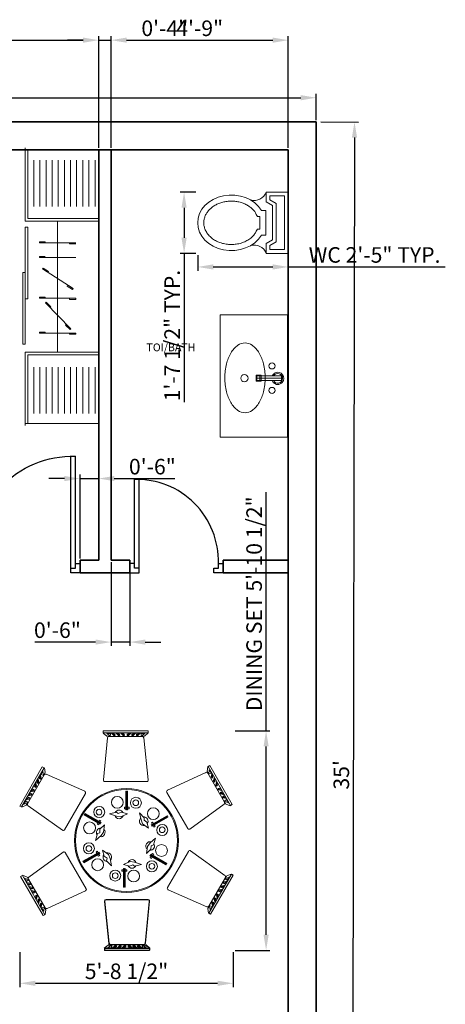
# Model space of a CAD drawing. Units: inches. Extents: x -24887 to 3061, y 1794 to 4919553.
# Tile 3 of 14: x 1777 to 1914, y 2047 to 2364. Entities that reach past the tile are written whole.
import ezdxf

# ---------------------------------------------------------------- set-up
doc = ezdxf.new("R2010")
doc.units = ezdxf.units.IN
for name, color, linetype, lineweight in [('A-ANNO-DIMS', 2, 'Continuous', 18), ('A-AREA-IDEN', 7, 'Continuous', 18), ('A-FLOR-FIXT', 9, 'Continuous', 18), ('A-FURN', 8, 'Continuous', 18), ('door', 4, 'Continuous', 25), ('wall', 7, 'Continuous', 35)]:
    doc.layers.add(name, color=color, linetype=linetype, lineweight=lineweight)
doc.styles.get("Standard").update_dxf_attribs({"font": 'arial.ttf'})
doc.dimstyles.new('ISO-25', dxfattribs={"dimtxt": 5, "dimasz": 5, "dimexe": 1.25, "dimexo": 0.625, "dimtad": 1, "dimdec": 1, "dimlunit": 3, "dimtxsty": 'Standard', "dimcen": 2.5, "dimadec": 0, "dimazin": 0, "dimtfac": 1, "dimtdec": 1, "dimtmove": 0, "dimatfit": 3, "dimfxl": 1, "dimarcsym": 0})

# ---------------------------------------------------------------- blocks, each defined once
blk = doc.blocks.new('A$C34930FF8')
at = {"ltscale": 0.05}
for p, q in [((0, 2252.4), (0, 16.8)), ((600, 2252.4), (0, 2252.4)), ((185.4, 1513), (185.4, 1521.5)), ((227.1, 1479.2), (233.2, 1485.2)), ((237.7, 1513), (237.7, 1521.5)), ((436.7, 1513), (436.7, 1504.4)), ((482.5, 1513), (482.5, 1504.4)), ((263.6, 1441.7), (269.7, 1447.7)), ((398.2, 1303.6), (392.1, 1297.6)), ((185.4, 1229.1), (185.4, 1237.7)), ((237.7, 1229.1), (237.7, 1237.7)), ((434.8, 1266.1), (428.7, 1260.1)), ((436.7, 1228.2), (436.7, 1219.7)), ((482.5, 1228.2), (482.5, 1219.7)), ((209.5, 1150.1), (214.1, 1157.3)), ((253.5, 1121.8), (258.1, 1129)), ((415.3, 1017.6), (410.6, 1010.5)), ((459.3, 989.3), (454.7, 982.1)), ((482.5, 894.9), (482.5, 886.3)), ((237.7, 775.3), (237.7, 783.9)), ((436.7, 775.3), (436.7, 766.8)), ((482.5, 775.3), (482.5, 766.8)), ((600, 16.8), (0, 16.8))]:
    blk.add_line(p, q, dxfattribs=at)
for p, q in [((580, 1690.9), (580, 2252.4)), ((600, 1669.3), (600, 2269.3)), ((30, 1790.9), (30, 2169.3)), ((80, 1790.9), (80, 2169.3)), ((130, 1790.9), (130, 2169.3)), ((180, 1790.9), (180, 2169.3)), ((230, 1790.9), (230, 2169.3)), ((280, 1790.9), (280, 2169.3)), ((330, 1790.9), (330, 2169.3)), ((380, 1790.9), (380, 2169.3)), ((430, 1790.9), (430, 2169.3)), ((480, 1790.9), (480, 2169.3)), ((530, 1790.9), (530, 2169.3)), ((580, 1690.9), (0, 1690.9)), ((600, 1669.3), (0, 1669.3)), ((335.4, 1666.1), (335.4, 603.1)), ((600, 1603.3), (620, 1603.3)), ((600, 1018.7), (600, 1603.3)), ((620, 1603.3), (620, 1018.7)), ((237.7, 1521.5), (185.4, 1521.5)), ((482.5, 1513), (185.4, 1513)), ((434.8, 1266.1), (227.4, 1478.9)), ((269.7, 1447.7), (233.2, 1485.2)), ((436.7, 1504.4), (482.5, 1504.4)), ((428.7, 1260.1), (392.1, 1297.6)), ((237.7, 1237.7), (185.4, 1237.7)), ((482.5, 1228.2), (185.4, 1228.2)), ((436.7, 1219.7), (482.5, 1219.7)), ((600, 1233.4), (580, 1233.4)), ((580, 1233.4), (580, 648.7)), ((600, 648.7), (600, 1233.4)), ((459.3, 989.3), (209.5, 1150.1)), ((258.1, 1129), (214.1, 1157.3)), ((454.7, 982.1), (410.6, 1010.5)), ((620, 1018.7), (600, 1018.7)), ((482.5, 894.9), (185.4, 894.9)), ((436.7, 886.3), (482.5, 886.3)), ((237.7, 783.9), (185.4, 783.9)), ((482.5, 775.3), (185.4, 775.3)), ((436.7, 766.8), (482.5, 766.8)), ((580, 648.7), (600, 648.7)), ((600, 600), (0, 600)), ((580, 578.3), (0, 578.3)), ((580, 578.3), (580, 16.8)), ((600, 600), (600, 0)), ((30, 478.3), (30, 100)), ((80, 478.3), (80, 100)), ((130, 478.3), (130, 100)), ((180, 478.3), (180, 100)), ((230, 478.3), (230, 100)), ((280, 478.3), (280, 100)), ((330, 478.3), (330, 100)), ((380, 478.3), (380, 100)), ((430, 478.3), (430, 100)), ((480, 478.3), (480, 100)), ((530, 478.3), (530, 100))]:
    blk.add_line(p, q)
blk = doc.blocks.new('A$C7C8779AE')
for p, q in [((0, 0.7405), (0, 0.5605)), ((0.5, 0.7405), (0, 0.7405)), ((0.5, 0.5605), (0.5, 0.7405)), ((0.47, 0.7105), (0.03, 0.7105)), ((0.03, 0.7105), (0.03, 0.5905)), ((0.47, 0.5905), (0.47, 0.7105)), ((0.03, 0.5905), (0.063, 0.5905)), ((0.093, 0.6405), (0.063, 0.5905)), ((0.11, 0.6105), (0.08, 0.5605)), ((0.093, 0.6405), (0.407, 0.6405)), ((0.11, 0.6105), (0.39, 0.6105)), ((0.42, 0.5605), (0.39, 0.6105)), ((0.437, 0.5905), (0.407, 0.6405)), ((0.437, 0.5905), (0.47, 0.5905)), ((0, 0.5605), (0.08, 0.5605)), ((0.1497, 0.557), (0.1497, 0.5203)), ((0.1497, 0.557), (0.3514, 0.557)), ((0.1997, 0.507), (0.1997, 0.4879)), ((0.1997, 0.507), (0.3014, 0.507)), ((0.3014, 0.507), (0.3014, 0.4879)), ((0.3514, 0.557), (0.3514, 0.5203)), ((0.42, 0.5605), (0.5, 0.5605))]:
    blk.add_line(p, q)
for centre, start, end in [((-0.0386, 0.4613), 344.64203, 68.73386), ((0.5386, 0.4613), 111.26614, 195.35797)]:
    blk.add_arc(centre, 0.1064, start, end)
blk.add_ellipse((0.2506, 0.2744), major_axis=(0, 0.2744), ratio=0.828948, start_param=0.459479, end_param=5.823706)
blk.add_open_spline([(0.1997, 0.4879), (0.1697, 0.474), (0.1642, 0.4702), (0.1512, 0.4602), (0.1438, 0.4535), (0.1298, 0.4388), (0.1233, 0.4306), (0.1111, 0.4131), (0.1055, 0.4037), (0.0956, 0.3838), (0.0912, 0.3733), (0.0838, 0.3516), (0.0808, 0.3403), (0.0762, 0.3172), (0.0746, 0.3055), (0.073, 0.2817), (0.0729, 0.2698), (0.0743, 0.246), (0.0758, 0.2342), (0.0801, 0.2111), (0.0831, 0.1998), (0.0903, 0.1779), (0.0945, 0.1673), (0.1043, 0.1473), (0.1098, 0.1378), (0.1218, 0.12), (0.1283, 0.1118), (0.1421, 0.0968), (0.1494, 0.09), (0.1646, 0.078), (0.1725, 0.0728), (0.1887, 0.064), (0.1969, 0.0603), (0.2137, 0.0547), (0.2222, 0.0527), (0.2392, 0.0502), (0.2478, 0.0498), (0.2664, 0.0505), (0.2764, 0.052), (0.2963, 0.0573), (0.3061, 0.061), (0.3253, 0.0707), (0.3346, 0.0766), (0.3525, 0.0906), (0.3611, 0.0987), (0.3771, 0.1169), (0.3845, 0.127), (0.3978, 0.1488), (0.4037, 0.1605), (0.4137, 0.1853), (0.4178, 0.1983), (0.424, 0.2251), (0.4261, 0.2389), (0.4282, 0.2668), (0.4283, 0.2809), (0.4262, 0.3088), (0.4241, 0.3226), (0.418, 0.3495), (0.414, 0.3625), (0.404, 0.3873), (0.3982, 0.3991), (0.385, 0.421), (0.3776, 0.4311), (0.3617, 0.4494), (0.3531, 0.4575), (0.3382, 0.4693), (0.3321, 0.4736), (0.3014, 0.4879)], degree=3, knots=[0.459479, 0.459479, 0.459479, 0.459479, 0.567422, 0.567422, 0.720865, 0.720865, 0.874307, 0.874307, 1.02775, 1.02775, 1.181192, 1.181192, 1.334635, 1.334635, 1.488077, 1.488077, 1.64152, 1.64152, 1.794963, 1.794963, 1.948405, 1.948405, 2.101848, 2.101848, 2.25529, 2.25529, 2.408733, 2.408733, 2.562175, 2.562175, 2.715618, 2.715618, 2.86906, 2.86906, 3.022503, 3.022503, 3.175946, 3.175946, 3.356457, 3.356457, 3.536968, 3.536968, 3.717479, 3.717479, 3.89799, 3.89799, 4.078501, 4.078501, 4.259012, 4.259012, 4.439523, 4.439523, 4.620035, 4.620035, 4.800546, 4.800546, 4.981057, 4.981057, 5.161568, 5.161568, 5.342079, 5.342079, 5.52259, 5.52259, 5.703101, 5.703101, 5.823706, 5.823706, 5.823706, 5.823706])
blk = doc.blocks.new('A$C50A015BB')
for p, q in [((0, 0.55), (1, 0.55)), ((0, 0.55), (0, 0)), ((0.4985, 0.5), (0.5385, 0.5)), ((0.4985, 0.5), (0.4985, 0.3)), ((0.5185, 0.5), (0.5185, 0.3)), ((0.5385, 0.5), (0.5385, 0.3)), ((1, 0.55), (1, 0)), ((0.4935, 0.335), (0.4935, 0.295)), ((0.4935, 0.335), (0.5435, 0.335)), ((0.4985, 0.325), (0.5385, 0.325)), ((0.5435, 0.335), (0.5435, 0.295)), ((0.4935, 0.295), (0.5435, 0.295)), ((0.4985, 0.3), (0.5385, 0.3)), ((0, 0), (1, 0)), ((0, 0), (1, 0))]:
    blk.add_line(p, q)
for centre, radius in [((0.4185, 0.424), 0.025), ((0.6185, 0.424), 0.025), ((0.5185, 0.1981), 0.0298)]:
    blk.add_circle(centre, radius)
for centre, radius, start, end in [((0.5201, 0.4703), 0.0497, 291.74253, 244.23308), ((0.5201, 0.4703), 0.0397, 297.63203, 237.02558), ((0.4772, 0.0383), 0.3252, 103.48533, 120.06859), ((0.5157, -0.1225), 0.4906, 90, 103.48533), ((0.5157, -0.1225), 0.4906, 76.51467, 90), ((0.5543, 0.0383), 0.3252, 59.93141, 76.51467), ((0.3299, 0.2031), 0.0991, 144.41781, 180), ((0.4185, 0.1397), 0.2081, 120.06859, 144.41781), ((0.613, 0.1397), 0.2081, 35.58219, 59.93141), ((0.7016, 0.2031), 0.0991, 0, 35.58219), ((0.3299, 0.2031), 0.0991, 180, 215.58219), ((0.7016, 0.2031), 0.0991, 324.41781, 0), ((0.4185, 0.2665), 0.2081, 215.58219, 239.93141), ((0.4772, 0.3679), 0.3252, 239.93141, 256.51467), ((0.5543, 0.3679), 0.3252, 283.48533, 300.06859), ((0.613, 0.2665), 0.2081, 300.06859, 324.41781), ((0.5157, 0.5288), 0.4906, 256.51467, 270), ((0.5157, 0.5288), 0.4906, 270, 283.48533)]:
    blk.add_arc(centre, radius, start, end)
blk = doc.blocks.new('A$C45501D90')
for p, q in [((-242, 1134), (224, 1134)), ((-242, 1113), (-242, 1134)), ((224, 1134), (224, 1113)), ((224, 1113), (-242, 1113)), ((-242, 1111), (-202, 1079)), ((-197, 1062), (-239, 628)), ((-204, 1106), (-166, 1108)), ((-169, 1081), (-204, 1106)), ((-202, 1079), (-169, 1081)), ((162, 1076), (-181, 1076)), ((-166, 1108), (-167, 1086)), ((-156, 1110), (-132, 1086)), ((-119, 1086), (-143, 1108)), ((-143, 1108), (-134, 1108)), ((-134, 1108), (-122, 1098)), ((-132, 1086), (-119, 1086)), ((-122, 1098), (-119, 1102)), ((-119, 1102), (-118, 1087)), ((-108, 1110), (-84, 1086)), ((-71, 1086), (-95, 1108)), ((-95, 1108), (-86, 1108)), ((-86, 1108), (-75, 1098)), ((-84, 1086), (-71, 1086)), ((-75, 1098), (-71, 1102)), ((-71, 1102), (-70, 1087)), ((-60, 1110), (-36, 1086)), ((-23, 1086), (-47, 1108)), ((-47, 1108), (-38, 1108)), ((-38, 1108), (-27, 1098)), ((-36, 1086), (-23, 1086)), ((-27, 1098), (-23, 1102)), ((-23, 1102), (-22, 1087)), ((8, 1102), (7, 1087)), ((8, 1086), (32, 1108)), ((12, 1098), (8, 1102)), ((21, 1086), (8, 1086)), ((23, 1108), (12, 1098)), ((45, 1110), (21, 1086)), ((32, 1108), (23, 1108)), ((56, 1102), (55, 1087)), ((56, 1086), (80, 1108)), ((60, 1098), (56, 1102)), ((69, 1086), (56, 1086)), ((71, 1108), (60, 1098)), ((93, 1110), (69, 1086)), ((80, 1108), (71, 1108)), ((104, 1102), (103, 1087)), ((104, 1086), (128, 1108)), ((107, 1098), (104, 1102)), ((117, 1086), (104, 1086)), ((119, 1108), (107, 1098)), ((141, 1110), (117, 1086)), ((128, 1108), (119, 1108)), ((189, 1106), (151, 1108)), ((151, 1108), (152, 1086)), ((154, 1081), (189, 1106)), ((187, 1079), (154, 1081)), ((225, 628), (178, 1062)), ((224, 1113), (187, 1079)), ((-1103, 357), (-870, 761)), ((-852, 750), (-1085, 347)), ((-864, 717), (-884, 684)), ((-870, 761), (-852, 750)), ((-859, 674), (-864, 717)), ((-849, 752), (-841, 702)), ((841, 765), (834, 715)), ((834, 715), (852, 687)), ((843, 766), (861, 776)), ((1076, 362), (843, 766)), ((852, 687), (856, 730)), ((856, 730), (877, 697)), ((861, 776), (1094, 373)), ((-851, 678), (-1023, 381)), ((-919, 624), (-924, 615)), ((-924, 615), (-921, 601)), ((-912, 592), (-919, 624)), ((-914, 635), (-906, 603)), ((-898, 642), (-902, 641)), ((-902, 641), (-890, 633)), ((-895, 665), (-900, 657)), ((-900, 657), (-898, 642)), ((-888, 633), (-895, 665)), ((-890, 677), (-882, 644)), ((-882, 644), (-888, 633)), ((-884, 684), (-864, 675)), ((-841, 702), (-859, 674)), ((-431, 509), (-831, 685)), ((821, 702), (424, 521)), ((1013, 398), (841, 695)), ((877, 697), (857, 688)), ((883, 690), (874, 657)), ((874, 657), (881, 646)), ((881, 646), (888, 678)), ((894, 654), (883, 646)), ((888, 678), (893, 670)), ((893, 670), (890, 655)), ((890, 655), (894, 654)), ((907, 648), (898, 616)), ((898, 616), (904, 605)), ((904, 605), (912, 637)), ((918, 613), (907, 604)), ((912, 637), (917, 628)), ((917, 628), (914, 614)), ((914, 614), (918, 613)), ((-991, 503), (-958, 511)), ((-952, 522), (-983, 513)), ((-983, 513), (-978, 521)), ((-978, 521), (-965, 526)), ((-965, 526), (-966, 530)), ((-966, 530), (-953, 525)), ((-958, 511), (-952, 522)), ((-945, 559), (-950, 558)), ((-950, 558), (-938, 550)), ((-943, 582), (-948, 574)), ((-948, 574), (-945, 559)), ((-936, 550), (-943, 582)), ((-938, 594), (-930, 561)), ((-930, 561), (-936, 550)), ((-921, 601), (-926, 600)), ((-926, 600), (-914, 591)), ((-906, 603), (-912, 592)), ((-223, 610), (209, 610)), ((931, 607), (922, 574)), ((922, 574), (928, 563)), ((928, 563), (936, 595)), ((942, 571), (931, 563)), ((936, 595), (941, 587)), ((941, 587), (938, 572)), ((938, 572), (942, 571)), ((951, 524), (944, 535)), ((944, 535), (976, 526)), ((958, 543), (945, 538)), ((983, 516), (951, 524)), ((957, 539), (958, 543)), ((971, 534), (957, 539)), ((976, 526), (971, 534)), ((-1060, 377), (-1042, 411)), ((-1042, 411), (-1024, 398)), ((-1039, 420), (-1006, 428)), ((-1000, 440), (-1031, 430)), ((-1031, 430), (-1026, 438)), ((-1026, 438), (-1012, 443)), ((-1015, 461), (-982, 470)), ((-1012, 443), (-1014, 448)), ((-1014, 448), (-1000, 442)), ((-976, 481), (-1007, 471)), ((-1007, 471), (-1002, 480)), ((-1006, 428), (-1000, 440)), ((-1002, 480), (-989, 485)), ((-989, 485), (-990, 489)), ((-990, 489), (-976, 483)), ((-982, 470), (-976, 481)), ((-640, 112), (-424, 486)), ((-6, 509, 91), (0, 509, 91)), ((-6, 318, 91), (-6, 509, 91)), ((0, 509, 91), (0, 318, 91)), ((6, 318, 91), (6, 509, 91)), ((6, 509, 91), (12, 509, 91)), ((12, 509, 91), (12, 318, 91)), ((417, 498), (633, 124)), ((968, 494), (1000, 484)), ((975, 483), (968, 494)), ((982, 502), (969, 496)), ((1007, 474), (975, 483)), ((981, 498), (982, 502)), ((995, 493), (981, 498)), ((999, 441), (992, 453)), ((992, 453), (1024, 443)), ((1006, 461), (993, 455)), ((1000, 484), (995, 493)), ((1031, 433), (999, 441)), ((1005, 456), (1006, 461)), ((1019, 451), (1005, 456)), ((1028, 377), (1013, 407)), ((1013, 407), (1053, 390)), ((1035, 424), (1016, 411)), ((1024, 443), (1019, 451)), ((1053, 390), (1035, 424)), ((-1085, 347), (-1103, 357)), ((-1083, 346), (-1036, 364)), ((-1020, 394), (-1060, 377)), ((-1036, 364), (-1020, 394)), ((-1018, 360), (-663, 107)), ((-22, 329, 91), (-22, 345, 91)), ((-22, 345, 91), (-6, 345, 91)), ((-6, 329, 91), (-22, 329, 91)), ((0, 318, 91), (-6, 318, 91)), ((0, 345, 91), (6, 345, 91)), ((6, 329, 91), (0, 329, 91)), ((12, 318, 91), (6, 318, 91)), ((12, 345, 91), (27, 345, 91)), ((27, 329, 91), (12, 329, 91)), ((27, 345, 91), (27, 329, 91)), ((656, 119), (1008, 377)), ((1076, 359), (1028, 377)), ((1094, 373), (1076, 362)), ((-436, 265, 91), (-433, 271, 91)), ((-271, 170, 91), (-436, 265, 91)), ((-433, 271, 91), (-268, 175, 91)), ((-431, 275, 91), (-428, 280, 91)), ((-265, 180, 91), (-431, 275, 91)), ((-428, 280, 91), (-262, 185, 91)), ((-286, 198, 91), (-278, 212, 91)), ((-278, 212, 91), (-264, 204, 91)), ((-264, 204, 91), (-272, 191, 91)), ((-175, 276, 91), (-105, 293, 91)), ((-103, 252, 91), (-175, 276, 91)), ((-105, 293, 91), (-86, 278, 91)), ((-60, 246, 91), (-103, 252, 91)), ((-86, 278, 91), (-52, 294, 91)), ((9, 276, 91), (-60, 246, 91)), ((-52, 294, 91), (9, 276, 91)), ((134, 288, 91), (184, 236, 91)), ((150, 214, 91), (134, 288, 91)), ((166, 173, 91), (150, 214, 91)), ((184, 236, 91), (181, 211, 91)), ((181, 211, 91), (211, 190, 91)), ((255, 162, 91), (421, 257, 91)), ((424, 252, 91), (258, 157, 91)), ((261, 152, 91), (426, 248, 91)), ((429, 242, 91), (264, 147, 91)), ((421, 257, 91), (424, 252, 91)), ((426, 248, 91), (429, 242, 91)), ((-303, 169, 91), (-294, 183, 91)), ((-289, 161, 91), (-303, 169, 91)), ((-291, 188, 91), (-289, 193, 91)), ((-281, 176, 91), (-289, 161, 91)), ((-275, 185, 91), (-278, 181, 91)), ((-277, 81, 91), (-274, 118, 91)), ((-274, 118, 91), (-227, 162, 91)), ((-268, 175, 91), (-271, 170, 91)), ((-262, 185, 91), (-265, 180, 91)), ((-227, 162, 91), (-236, 87, 91)), ((227, 128, 91), (166, 173, 91)), ((211, 190, 91), (227, 128, 91)), ((258, 157, 91), (255, 162, 91)), ((257, 182, 91), (270, 190, 91)), ((265, 168, 91), (257, 182, 91)), ((264, 147, 91), (261, 152, 91)), ((271, 158, 91), (268, 162, 91)), ((270, 190, 91), (278, 175, 91)), ((281, 139, 91), (274, 153, 91)), ((281, 170, 91), (284, 165, 91)), ((295, 147, 91), (281, 139, 91)), ((287, 160, 91), (295, 147, 91)), ((-320, 2, 91), (-299, 72, 91)), ((-263, 53, 91), (-320, 2, 91)), ((-299, 72, 91), (-277, 81, 91)), ((-236, 87, 91), (-263, 53, 91)), ((243, -25, 91), (299, 26, 91)), ((299, 26, 91), (279, -44, 91)), ((-247, -100, 91), (-187, -145, 91)), ((-232, -162, 91), (-247, -100, 91)), ((207, -134, 91), (216, -60, 91)), ((253, -90, 91), (207, -134, 91)), ((216, -60, 91), (243, -25, 91)), ((256, -53, 91), (253, -90, 91)), ((279, -44, 91), (256, -53, 91)), ((-656, -119), (-1008, -377)), ((-417, -498), (-633, -124)), ((-450, -214, 91), (-284, -119, 91)), ((-281, -124, 91), (-447, -220, 91)), ((-444, -224, 91), (-279, -129, 91)), ((-276, -134, 91), (-441, -229, 91)), ((-315, -119, 91), (-302, -111, 91)), ((-307, -132, 91), (-315, -119, 91)), ((-302, -142, 91), (-304, -137, 91)), ((-302, -111, 91), (-294, -125, 91)), ((-290, -162, 91), (-299, -147, 91)), ((-291, -130, 91), (-288, -134, 91)), ((-277, -154, 91), (-290, -162, 91)), ((-285, -140, 91), (-277, -154, 91)), ((-284, -119, 91), (-281, -124, 91)), ((-279, -129, 91), (-276, -134, 91)), ((-201, -183, 91), (-232, -162, 91)), ((-205, -208, 91), (-201, -183, 91)), ((-187, -145, 91), (-170, -186, 91)), ((-170, -186, 91), (-155, -260, 91)), ((242, -157, 91), (245, -152, 91)), ((407, -252, 91), (242, -157, 91)), ((244, -176, 91), (252, -163, 91)), ((257, -184, 91), (244, -176, 91)), ((245, -152, 91), (410, -247, 91)), ((248, -147, 91), (251, -142, 91)), ((413, -243, 91), (248, -147, 91)), ((251, -142, 91), (416, -237, 91)), ((255, -157, 91), (257, -153, 91)), ((265, -170, 91), (257, -184, 91)), ((260, -148, 91), (269, -133, 91)), ((271, -160, 91), (268, -165, 91)), ((269, -133, 91), (282, -141, 91)), ((282, -141, 91), (274, -155, 91)), ((640, -112), (424, -486)), ((1018, -360), (663, -107)), ((-447, -220, 91), (-450, -214, 91)), ((-441, -229, 91), (-444, -224, 91)), ((-155, -260, 91), (-205, -208, 91)), ((-48, -317, 91), (-48, -301, 91)), ((-48, -301, 91), (-32, -301, 91)), ((-32, -481, 91), (-32, -290, 91)), ((-32, -290, 91), (-26, -290, 91)), ((-30, -248, 91), (39, -218, 91)), ((32, -266, 91), (-30, -248, 91)), ((-26, -290, 91), (-26, -481, 91)), ((-26, -301, 91), (-21, -301, 91)), ((-21, -481, 91), (-21, -290, 91)), ((-21, -290, 91), (-15, -290, 91)), ((-15, -290, 91), (-15, -481, 91)), ((-15, -301, 91), (2, -301, 91)), ((2, -301, 91), (2, -317, 91)), ((65, -250, 91), (32, -266, 91)), ((39, -218, 91), (83, -224, 91)), ((84, -265, 91), (65, -250, 91)), ((83, -224, 91), (155, -248, 91)), ((155, -248, 91), (84, -265, 91)), ((410, -247, 91), (407, -252, 91)), ((416, -237, 91), (413, -243, 91)), ((-1094, -373), (-1076, -362)), ((-861, -776), (-1094, -373)), ((-1076, -359), (-1028, -377)), ((-1076, -362), (-843, -766)), ((-1053, -390), (-1035, -424)), ((-1013, -407), (-1053, -390)), ((-1028, -377), (-1013, -407)), ((-1013, -398), (-841, -695)), ((-32, -317, 91), (-48, -317, 91)), ((-21, -317, 91), (-26, -317, 91)), ((2, -317, 91), (-15, -317, 91)), ((851, -678), (1023, -381)), ((852, -750), (1085, -347)), ((1103, -357), (870, -761)), ((1036, -364), (1020, -394)), ((1020, -394), (1060, -377)), ((1042, -411), (1024, -398)), ((1083, -346), (1036, -364)), ((1060, -377), (1042, -411)), ((1085, -347), (1103, -357)), ((-1035, -424), (-1016, -411)), ((-1031, -433), (-999, -441)), ((-1024, -443), (-1019, -451)), ((-992, -453), (-1024, -443)), ((-1019, -451), (-1005, -456)), ((-1007, -474), (-975, -483)), ((-1006, -461), (-993, -455)), ((-1005, -456), (-1006, -461)), ((-968, -494), (-1000, -484)), ((-1000, -484), (-995, -493)), ((-999, -441), (-992, -453)), ((-995, -493), (-981, -498)), ((-982, -502), (-969, -496)), ((-981, -498), (-982, -502)), ((-975, -483), (-968, -494)), ((-26, -481, 91), (-32, -481, 91)), ((-15, -481, 91), (-21, -481, 91)), ((991, -503), (958, -511)), ((982, -470), (976, -481)), ((976, -481), (1007, -471)), ((990, -489), (976, -483)), ((1015, -461), (982, -470)), ((1002, -480), (989, -485)), ((989, -485), (990, -489)), ((1006, -428), (1000, -440)), ((1000, -440), (1031, -430)), ((1014, -448), (1000, -442)), ((1007, -471), (1002, -480)), ((1039, -420), (1006, -428)), ((1026, -438), (1012, -443)), ((1012, -443), (1014, -448)), ((1031, -430), (1026, -438)), ((-983, -516), (-951, -524)), ((-944, -535), (-976, -526)), ((-976, -526), (-971, -534)), ((-971, -534), (-957, -539)), ((-958, -543), (-945, -538)), ((-957, -539), (-958, -543)), ((-951, -524), (-944, -535)), ((-942, -571), (-931, -563)), ((-938, -572), (-942, -571)), ((-941, -587), (-938, -572)), ((-936, -595), (-941, -587)), ((-928, -563), (-936, -595)), ((-931, -607), (-922, -574)), ((-922, -574), (-928, -563)), ((-918, -613), (-907, -604)), ((-904, -605), (-912, -637)), ((-898, -616), (-904, -605)), ((-821, -702), (-424, -521)), ((223, -610), (-209, -610)), ((431, -509), (831, -685)), ((906, -603), (912, -592)), ((914, -635), (906, -603)), ((912, -592), (919, -624)), ((926, -600), (914, -591)), ((921, -601), (926, -600)), ((924, -615), (921, -601)), ((930, -561), (936, -550)), ((938, -594), (930, -561)), ((936, -550), (943, -582)), ((950, -558), (938, -550)), ((943, -582), (948, -574)), ((945, -559), (950, -558)), ((948, -574), (945, -559)), ((958, -511), (952, -522)), ((952, -522), (983, -513)), ((966, -530), (953, -525)), ((978, -521), (965, -526)), ((965, -526), (966, -530)), ((983, -513), (978, -521)), ((-914, -614), (-918, -613)), ((-917, -628), (-914, -614)), ((-912, -637), (-917, -628)), ((-907, -648), (-898, -616)), ((-894, -654), (-883, -646)), ((-890, -655), (-894, -654)), ((-893, -670), (-890, -655)), ((-888, -678), (-893, -670)), ((-881, -646), (-888, -678)), ((-883, -690), (-874, -657)), ((-874, -657), (-881, -646)), ((-877, -697), (-857, -688)), ((-856, -730), (-877, -697)), ((-852, -687), (-856, -730)), ((-834, -715), (-852, -687)), ((-229, -629), (-182, -1063)), ((-225, -628), (-178, -1062)), ((219, -612), (-213, -612)), ((193, -1063), (235, -629)), ((197, -1062), (239, -628)), ((841, -702), (859, -674)), ((849, -752), (841, -702)), ((859, -674), (864, -717)), ((884, -684), (864, -675)), ((864, -717), (884, -684)), ((882, -644), (888, -633)), ((890, -677), (882, -644)), ((888, -633), (895, -665)), ((902, -641), (890, -633)), ((895, -665), (900, -657)), ((898, -642), (902, -641)), ((900, -657), (898, -642)), ((919, -624), (924, -615)), ((-843, -766), (-861, -776)), ((-841, -765), (-834, -715)), ((870, -761), (852, -750)), ((-231, -1113), (-191, -1081)), ((-228, -1114), (238, -1114)), ((-228, -1135), (-228, -1114)), ((-227, -1111), (-187, -1079)), ((-224, -1113), (242, -1113)), ((-224, -1134), (-224, -1113)), ((-158, -1082), (-193, -1108)), ((-193, -1108), (-155, -1109)), ((-191, -1081), (-158, -1082)), ((-154, -1081), (-189, -1106)), ((-189, -1106), (-151, -1108)), ((-187, -1079), (-154, -1081)), ((-166, -1078), (177, -1078)), ((-162, -1076), (181, -1076)), ((-155, -1109), (-156, -1087)), ((-151, -1108), (-152, -1086)), ((-145, -1111), (-121, -1087)), ((-141, -1110), (-117, -1086)), ((-108, -1087), (-132, -1109)), ((-132, -1109), (-123, -1109)), ((-104, -1086), (-128, -1108)), ((-128, -1108), (-119, -1108)), ((-123, -1109), (-112, -1100)), ((-121, -1087), (-108, -1087)), ((-119, -1108), (-107, -1098)), ((-117, -1086), (-104, -1086)), ((-112, -1100), (-108, -1103)), ((-108, -1103), (-107, -1089)), ((-107, -1098), (-104, -1102)), ((-104, -1102), (-103, -1087)), ((-97, -1111), (-73, -1087)), ((-93, -1110), (-69, -1086)), ((-60, -1087), (-84, -1109)), ((-84, -1109), (-75, -1109)), ((-56, -1086), (-80, -1108)), ((-80, -1108), (-71, -1108)), ((-75, -1109), (-64, -1100)), ((-73, -1087), (-60, -1087)), ((-71, -1108), (-60, -1098)), ((-69, -1086), (-56, -1086)), ((-64, -1100), (-60, -1103)), ((-60, -1103), (-59, -1089)), ((-60, -1098), (-56, -1102)), ((-56, -1102), (-55, -1087)), ((-49, -1111), (-25, -1087)), ((-45, -1110), (-21, -1086)), ((-13, -1087), (-37, -1109)), ((-37, -1109), (-27, -1109)), ((-8, -1086), (-32, -1108)), ((-32, -1108), (-23, -1108)), ((-27, -1109), (-16, -1100)), ((-25, -1087), (-13, -1087)), ((-23, -1108), (-12, -1098)), ((-21, -1086), (-8, -1086)), ((-16, -1100), (-13, -1103)), ((-13, -1103), (-11, -1089)), ((-12, -1098), (-8, -1102)), ((-8, -1102), (-7, -1087)), ((19, -1103), (18, -1089)), ((19, -1087), (43, -1109)), ((32, -1087), (19, -1087)), ((23, -1100), (19, -1103)), ((23, -1102), (22, -1087)), ((23, -1086), (47, -1108)), ((36, -1086), (23, -1086)), ((27, -1098), (23, -1102)), ((34, -1109), (23, -1100)), ((38, -1108), (27, -1098)), ((56, -1111), (32, -1087)), ((43, -1109), (34, -1109)), ((60, -1110), (36, -1086)), ((47, -1108), (38, -1108)), ((67, -1103), (66, -1089)), ((67, -1087), (91, -1109)), ((80, -1087), (67, -1087)), ((70, -1100), (67, -1103)), ((71, -1102), (70, -1087)), ((82, -1109), (70, -1100)), ((71, -1086), (95, -1108)), ((84, -1086), (71, -1086)), ((75, -1098), (71, -1102)), ((86, -1108), (75, -1098)), ((104, -1111), (80, -1087)), ((91, -1109), (82, -1109)), ((108, -1110), (84, -1086)), ((95, -1108), (86, -1108)), ((115, -1103), (114, -1089)), ((115, -1087), (139, -1109)), ((128, -1087), (115, -1087)), ((118, -1100), (115, -1103)), ((119, -1102), (118, -1087)), ((130, -1109), (118, -1100)), ((119, -1086), (143, -1108)), ((132, -1086), (119, -1086)), ((122, -1098), (119, -1102)), ((134, -1108), (122, -1098)), ((152, -1111), (128, -1087)), ((139, -1109), (130, -1109)), ((156, -1110), (132, -1086)), ((143, -1108), (134, -1108)), ((161, -1109), (163, -1087)), ((200, -1108), (161, -1109)), ((198, -1081), (165, -1082)), ((165, -1082), (200, -1108)), ((166, -1108), (167, -1086)), ((204, -1106), (166, -1108)), ((202, -1079), (169, -1081)), ((169, -1081), (204, -1106)), ((238, -1113), (198, -1081)), ((242, -1111), (202, -1079)), ((238, -1114), (238, -1135)), ((242, -1113), (242, -1134)), ((238, -1135), (-228, -1135)), ((242, -1134), (-224, -1134))]:
    blk.add_line(p, q)
for centre, radius in [((0, 0), 537), ((0, 0), 527), ((-95, 395, 91), 61.3), ((97, 390, 91), 56.9), ((96, 391, 91), 29.4), ((-282, 295, 91), 56.9), ((-284, 294, 91), 29.4), ((277, 278, 91), 61.3), ((-382, 131, 91), 61.3), ((369, 109, 91), 56.9), ((369, 111, 91), 29.4), ((-389, -81, 91), 56.9), ((-389, -83, 91), 29.4), ((362, -103, 91), 61.3), ((-298, -250, 91), 61.3), ((-117, -362, 91), 56.9), ((262, -267, 91), 56.9), ((263, -266, 91), 29.4), ((-116, -363, 91), 29.4), ((74, -367, 91), 61.3)]:
    blk.add_circle(centre, radius)
for centre, radius, start, end in [((-181, 1060), 16, 90, 174.5199), ((162, 1060), 16, 6.2572, 90), ((-837, 670), 16, 66.2572, 150), ((-223, 626), 16, 174.5199, 270), ((209, 626), 16, 270, 6.2572), ((827, 687), 16, 30, 114.5199), ((-438, 494), 16, 330, 66.2572), ((431, 506), 16, 114.5199, 210), ((-1009, 373), 16, 150, 234.5199), ((-77, 270, 91), 44.6, 25.8558, 153.3359), ((999, 390), 16, 306.2572, 30), ((-77, 270, 91), 44.6, 195.9338, 342.9389), ((178, 200, 91), 44.6, 135.9338, 282.9389), ((178, 200, 91), 44.6, 325.8558, 93.3359), ((-654, 120), 16, 234.5199, 330), ((-266, 84, 91), 44.6, 85.8558, 213.3359), ((-266, 84, 91), 44.6, 255.9338, 42.9389), ((647, 132), 16, 210, 306.2572), ((245, -56, 91), 44.6, 75.9338, 222.9389), ((245, -56, 91), 44.6, 265.8558, 33.3359), ((-647, -132), 16, 30, 126.2572), ((-198, -172, 91), 44.6, 145.8558, 273.3359), ((-198, -172, 91), 44.6, 315.9338, 102.9389), ((57, -242, 91), 44.6, 15.9338, 162.9389), ((654, -120), 16, 54.5199, 150), ((57, -242, 91), 44.6, 205.8558, 333.3359), ((-999, -390), 16, 126.2572, 210), ((1009, -373), 16, 330, 54.5199), ((-431, -506), 16, 294.5199, 30), ((438, -494), 16, 150, 246.2572), ((-209, -626), 16, 90, 186.2572), ((223, -626), 16, 354.5199, 90), ((-827, -687), 16, 210, 294.5199), ((-213, -628), 16, 90, 186.2572), ((219, -628), 16, 354.5199, 90), ((837, -670), 16, 246.2572, 330), ((-166, -1062), 16, 186.2572, 270), ((-162, -1060), 16, 186.2572, 270), ((177, -1062), 16, 270, 354.5199), ((181, -1060), 16, 270, 354.5199)]:
    blk.add_arc(centre, radius, start, end)
blk = doc.blocks.new('*D28')
at = {"layer": 'A-ANNO-DIMS', "color": 0, "lineweight": -2, "transparency": 16777216}
for p, q in [((1608.43, 2331.48), (1608.43, 2339.9)), ((1613.43, 2338.65), (1867.43, 2338.65)), ((1872.43, 2331.48), (1872.43, 2339.9))]:
    blk.add_line(p, q, dxfattribs=at)
at = {"layer": 'A-ANNO-DIMS', "color": 0, "transparency": 16777216}
for points in [[(1613.43, 2339.48), (1613.43, 2337.81), (1608.43, 2338.65)], [(1867.43, 2339.48), (1867.43, 2337.81), (1872.43, 2338.65)]]:
    blk.add_solid(points, dxfattribs=at)
at = {"layer": 'Defpoints', "color": 0, "transparency": 16777216}
for p in [(1872.43, 2338.65), (1608.43, 2330.86), (1872.43, 2330.86)]:
    blk.add_point(p, dxfattribs=at)
at = {"layer": 'A-ANNO-DIMS', "color": 0, "transparency": 16777216, "insert": (1740.43, 2341.78), "char_height": 5, "attachment_point": 5}
blk.add_mtext("22'", dxfattribs=at)
blk = doc.blocks.new('*D29')
at = {"layer": 'A-ANNO-DIMS', "color": 0, "lineweight": -2, "transparency": 16777216}
for p, q in [((1873.91, 2330.86), (1885.98, 2330.83)), ((1884.72, 2325.84), (1883.89, 1915.84)), ((1873.06, 1910.86), (1885.13, 1910.83))]:
    blk.add_line(p, q, dxfattribs=at)
at = {"layer": 'A-ANNO-DIMS', "color": 0, "transparency": 16777216}
for points in [[(1883.89, 2325.84), (1885.56, 2325.83), (1884.73, 2330.84)], [(1883.05, 1915.84), (1884.72, 1915.83), (1883.88, 1910.84)]]:
    blk.add_solid(points, dxfattribs=at)
at = {"layer": 'Defpoints', "color": 0, "transparency": 16777216}
for p in [(1873.29, 2330.86), (1872.43, 1910.86), (1883.88, 1910.84)]:
    blk.add_point(p, dxfattribs=at)
at = {"layer": 'A-ANNO-DIMS', "color": 0, "transparency": 16777216, "insert": (1881.13, 2120.84), "char_height": 5, "attachment_point": 5, "rotation": 89.8832}
blk.add_mtext("35'", dxfattribs=at)
blk = doc.blocks.new('DOOR-SINGLE-36IN')
for p, q in [((34.5, 36), (37.5, 36)), ((34.5, 34.5), (34.5, 36)), ((37.5, 36), (37.5, 33)), ((36, 34.5), (34.5, 34.5)), ((36, 33), (36, 34.5)), ((37.5, 33), (36, 33)), ((36, 3), (0, 3)), ((36, 1.5), (0, 1.5)), ((36, 1.5), (34.5, 1.5)), ((34.5, 1.5), (34.5, 0)), ((34.5, 0), (37.5, 0)), ((37.5, 3), (36, 3)), ((36, 3), (36, 1.5)), ((37.5, 0), (37.5, 3))]:
    blk.add_line(p, q)
blk.add_arc((32.32, 2.25), 32.32, 86.1244, 181.3295)
blk = doc.blocks.new('DOOR-SINGLE-30IN')
for p, q in [((1.5, 1.5), (1.5, 30)), ((3, 0), (3, 30)), ((0, 3), (0, 0)), ((1.5, 3), (0, 3)), ((0, 0), (3, 0)), ((1.5, 1.5), (1.5, 3)), ((3, 1.5), (1.5, 1.5)), ((3, 0), (3, 1.5)), ((27, 0), (27, 1.5)), ((27, 1.5), (28.5, 1.5)), ((30, 0), (27, 0)), ((28.5, 1.5), (28.5, 3)), ((28.5, 3), (30, 3)), ((30, 3), (30, 0))]:
    blk.add_line(p, q)
blk.add_arc((2.25, 3.75), 26.26, 358.3634, 91.6366)
blk = doc.blocks.new('*D44')
at = {"layer": 'A-ANNO-DIMS', "color": 0, "lineweight": -2, "transparency": 16777216}
for p, q in [((1834.28, 2287.97), (1834.28, 2282.97)), ((1863.43, 2287.97), (1863.43, 2282.97)), ((1839.28, 2284.22), (1858.43, 2284.22)), ((1863.43, 2284.22), (1913.94, 2284.22))]:
    blk.add_line(p, q, dxfattribs=at)
at = {"layer": 'A-ANNO-DIMS', "color": 0, "transparency": 16777216}
for points in [[(1839.28, 2285.05), (1839.28, 2283.39), (1834.28, 2284.22)], [(1858.43, 2285.05), (1858.43, 2283.39), (1863.43, 2284.22)]]:
    blk.add_solid(points, dxfattribs=at)
at = {"layer": 'Defpoints', "color": 0, "transparency": 16777216}
for p in [(1834.28, 2288.59), (1863.43, 2288.59), (1863.43, 2284.22)]:
    blk.add_point(p, dxfattribs=at)
at = {"layer": 'A-ANNO-DIMS', "color": 0, "transparency": 16777216, "insert": (1891.19, 2287.43), "char_height": 5, "attachment_point": 5}
blk.add_mtext('WC 2\'-5" TYP.', dxfattribs=at)
blk = doc.blocks.new('*D45')
at = {"layer": 'A-ANNO-DIMS', "color": 0, "lineweight": -2, "transparency": 16777216}
for p, q in [((1833.65, 2308.28), (1828.66, 2308.28)), ((1829.91, 2303.28), (1829.91, 2293.59)), ((1833.65, 2288.59), (1828.66, 2288.59)), ((1829.91, 2288.59), (1829.91, 2240.68))]:
    blk.add_line(p, q, dxfattribs=at)
at = {"layer": 'A-ANNO-DIMS', "color": 0, "transparency": 16777216}
for points in [[(1829.07, 2303.28), (1830.74, 2303.28), (1829.91, 2308.28)], [(1829.07, 2293.59), (1830.74, 2293.59), (1829.91, 2288.59)]]:
    blk.add_solid(points, dxfattribs=at)
at = {"layer": 'Defpoints', "color": 0, "transparency": 16777216}
for p in [(1834.28, 2308.28), (1829.91, 2288.59), (1834.28, 2288.59)]:
    blk.add_point(p, dxfattribs=at)
at = {"layer": 'A-ANNO-DIMS', "color": 0, "transparency": 16777216, "insert": (1826.7, 2262.14), "char_height": 5, "attachment_point": 5, "rotation": 90}
blk.add_mtext('1\'-7 1/2" TYP.', dxfattribs=at)
blk = doc.blocks.new('*D50')
at = {"layer": 'A-ANNO-DIMS', "color": 0, "lineweight": -2, "transparency": 16777216}
for p, q in [((1856.29, 2135), (1856.29, 2211.74)), ((1846.33, 2135), (1857.54, 2135)), ((1856.29, 2069.4), (1856.29, 2130)), ((1846.33, 2064.4), (1857.54, 2064.4))]:
    blk.add_line(p, q, dxfattribs=at)
at = {"layer": 'A-ANNO-DIMS', "color": 0, "transparency": 16777216}
for points in [[(1855.46, 2130), (1857.12, 2130), (1856.29, 2135)], [(1855.46, 2069.4), (1857.12, 2069.4), (1856.29, 2064.4)]]:
    blk.add_solid(points, dxfattribs=at)
at = {"layer": 'Defpoints', "color": 0, "transparency": 16777216}
for p in [(1845.7, 2135), (1856.29, 2135), (1845.7, 2064.4)]:
    blk.add_point(p, dxfattribs=at)
at = {"layer": 'A-ANNO-DIMS', "color": 0, "transparency": 16777216, "insert": (1853.08, 2175.87), "char_height": 5, "attachment_point": 5, "rotation": 90}
blk.add_mtext('DINING SET 5\'-10 1/2"', dxfattribs=at)
blk = doc.blocks.new('*D51')
at = {"layer": 'A-ANNO-DIMS', "color": 0, "lineweight": -2, "transparency": 16777216}
for p, q in [((1777.06, 2063.77), (1777.06, 2052.56)), ((1845.7, 2063.77), (1845.7, 2052.56)), ((1782.06, 2053.81), (1840.7, 2053.81))]:
    blk.add_line(p, q, dxfattribs=at)
at = {"layer": 'A-ANNO-DIMS', "color": 0, "transparency": 16777216}
for points in [[(1782.06, 2054.64), (1782.06, 2052.97), (1777.06, 2053.81)], [(1840.7, 2054.64), (1840.7, 2052.97), (1845.7, 2053.81)]]:
    blk.add_solid(points, dxfattribs=at)
at = {"layer": 'Defpoints', "color": 0, "transparency": 16777216}
for p in [(1777.06, 2064.4), (1845.7, 2064.4), (1845.7, 2053.81)]:
    blk.add_point(p, dxfattribs=at)
at = {"layer": 'A-ANNO-DIMS', "color": 0, "transparency": 16777216, "insert": (1811.38, 2057.02), "char_height": 5, "attachment_point": 5}
blk.add_mtext('5\'-8 1/2"', dxfattribs=at)
blk = doc.blocks.new('*D67')
at = {"layer": 'A-ANNO-DIMS', "color": 0, "lineweight": -2, "transparency": 16777216}
for p, q in [((1617.43, 2322.48), (1617.43, 2358.41)), ((1622.43, 2357.16), (1797.43, 2357.16)), ((1802.43, 2322.48), (1802.43, 2358.41))]:
    blk.add_line(p, q, dxfattribs=at)
at = {"layer": 'A-ANNO-DIMS', "color": 0, "transparency": 16777216}
for points in [[(1622.43, 2357.99), (1622.43, 2356.33), (1617.43, 2357.16)], [(1797.43, 2357.99), (1797.43, 2356.33), (1802.43, 2357.16)]]:
    blk.add_solid(points, dxfattribs=at)
at = {"layer": 'Defpoints', "color": 0, "transparency": 16777216}
for p in [(1802.43, 2357.16), (1617.43, 2321.86), (1802.43, 2321.86)]:
    blk.add_point(p, dxfattribs=at)
at = {"layer": 'A-ANNO-DIMS', "color": 0, "transparency": 16777216, "insert": (1709.93, 2360.34), "char_height": 5, "attachment_point": 5}
blk.add_mtext('15\'-5"', dxfattribs=at)
blk = doc.blocks.new('*D68')
at = {"layer": 'A-ANNO-DIMS', "color": 0, "lineweight": -2, "transparency": 16777216}
for p, q in [((1797.43, 2357.16), (1792.43, 2357.16)), ((1802.43, 2322.48), (1802.43, 2358.41)), ((1802.43, 2357.16), (1806.43, 2357.16)), ((1806.43, 2322.48), (1806.43, 2358.41)), ((1811.43, 2357.16), (1830.97, 2357.16))]:
    blk.add_line(p, q, dxfattribs=at)
at = {"layer": 'A-ANNO-DIMS', "color": 0, "transparency": 16777216}
for points in [[(1797.43, 2357.99), (1797.43, 2356.33), (1802.43, 2357.16)], [(1811.43, 2357.99), (1811.43, 2356.33), (1806.43, 2357.16)]]:
    blk.add_solid(points, dxfattribs=at)
at = {"layer": 'Defpoints', "color": 0, "transparency": 16777216}
for p in [(1806.43, 2357.16), (1802.43, 2321.86), (1806.43, 2321.86)]:
    blk.add_point(p, dxfattribs=at)
at = {"layer": 'A-ANNO-DIMS', "color": 0, "transparency": 16777216, "insert": (1823.7, 2360.34), "char_height": 5, "attachment_point": 5}
blk.add_mtext('0\'-4"', dxfattribs=at)
blk = doc.blocks.new('*D69')
at = {"layer": 'A-ANNO-DIMS', "color": 0, "lineweight": -2, "transparency": 16777216}
for p, q in [((1806.43, 2322.48), (1806.43, 2358.41)), ((1811.43, 2357.16), (1858.43, 2357.16)), ((1863.43, 2322.48), (1863.43, 2358.41))]:
    blk.add_line(p, q, dxfattribs=at)
at = {"layer": 'A-ANNO-DIMS', "color": 0, "transparency": 16777216}
for points in [[(1811.43, 2357.99), (1811.43, 2356.33), (1806.43, 2357.16)], [(1858.43, 2357.99), (1858.43, 2356.33), (1863.43, 2357.16)]]:
    blk.add_solid(points, dxfattribs=at)
at = {"layer": 'Defpoints', "color": 0, "transparency": 16777216}
for p in [(1863.43, 2357.16), (1806.43, 2321.86), (1863.43, 2321.86)]:
    blk.add_point(p, dxfattribs=at)
at = {"layer": 'A-ANNO-DIMS', "color": 0, "transparency": 16777216, "insert": (1834.93, 2360.34), "char_height": 5, "attachment_point": 5}
blk.add_mtext('4\'-9"', dxfattribs=at)
blk = doc.blocks.new('*D79')
at = {"layer": 'A-ANNO-DIMS', "color": 0, "lineweight": -2, "transparency": 16777216}
for p, q in [((1796.43, 2190.48), (1796.43, 2217.41)), ((1802.43, 2190.48), (1802.43, 2217.41)), ((1791.43, 2216.16), (1786.43, 2216.16)), ((1796.43, 2216.16), (1802.43, 2216.16)), ((1807.43, 2216.16), (1826.97, 2216.16))]:
    blk.add_line(p, q, dxfattribs=at)
at = {"layer": 'A-ANNO-DIMS', "color": 0, "transparency": 16777216}
for points in [[(1791.43, 2216.99), (1791.43, 2215.33), (1796.43, 2216.16)], [(1807.43, 2216.99), (1807.43, 2215.33), (1802.43, 2216.16)]]:
    blk.add_solid(points, dxfattribs=at)
at = {"layer": 'Defpoints', "color": 0, "transparency": 16777216}
for p in [(1802.43, 2216.16), (1796.43, 2189.86), (1802.43, 2189.86)]:
    blk.add_point(p, dxfattribs=at)
at = {"layer": 'A-ANNO-DIMS', "color": 0, "transparency": 16777216, "insert": (1819.7, 2219.34), "char_height": 5, "attachment_point": 5}
blk.add_mtext('0\'-6"', dxfattribs=at)
blk = doc.blocks.new('*D80')
at = {"layer": 'A-ANNO-DIMS', "color": 0, "lineweight": -2, "transparency": 16777216}
for p, q in [((1806.43, 2189.23), (1806.43, 2162.31)), ((1812.43, 2189.23), (1812.43, 2162.31)), ((1801.43, 2163.56), (1781.89, 2163.56)), ((1812.43, 2163.56), (1806.43, 2163.56)), ((1817.43, 2163.56), (1822.43, 2163.56))]:
    blk.add_line(p, q, dxfattribs=at)
at = {"layer": 'A-ANNO-DIMS', "color": 0, "transparency": 16777216}
for points in [[(1801.43, 2164.39), (1801.43, 2162.73), (1806.43, 2163.56)], [(1817.43, 2164.39), (1817.43, 2162.73), (1812.43, 2163.56)]]:
    blk.add_solid(points, dxfattribs=at)
at = {"layer": 'Defpoints', "color": 0, "transparency": 16777216}
for p in [(1806.43, 2189.86), (1812.43, 2189.86), (1806.43, 2163.56)]:
    blk.add_point(p, dxfattribs=at)
at = {"layer": 'A-ANNO-DIMS', "color": 0, "transparency": 16777216, "insert": (1789.16, 2166.74), "char_height": 5, "attachment_point": 5}
blk.add_mtext('0\'-6"', dxfattribs=at)

msp = doc.modelspace()

# ---------------------------------------------------------------- linework, layer by layer
at = {"layer": 'wall'}
for p, q in [((1872.43, 2330.86), (1608.43, 2330.86)), ((1872.43, 1910.86), (1872.43, 2330.86)), ((1863.43, 2321.86), (1617.43, 2321.86)), ((1802.43, 2321.86), (1802.43, 2189.86)), ((1806.43, 2321.86), (1806.43, 2189.86)), ((1863.43, 1919.86), (1863.43, 2321.86)), ((1802.43, 2189.86), (1796.43, 2189.86)), ((1796.43, 2189.86), (1796.43, 2185.86)), ((1812.43, 2189.86), (1806.43, 2189.86)), ((1812.43, 2189.86), (1812.43, 2185.86)), ((1863.43, 2189.86), (1842.43, 2189.86)), ((1842.43, 2189.86), (1842.43, 2185.86)), ((1812.43, 2185.86), (1796.43, 2185.86)), ((1863.43, 2185.86), (1842.43, 2185.86))]:
    msp.add_line(p, q, dxfattribs=at)

# ---------------------------------------------------------------- block references
at = {"layer": 'A-FLOR-FIXT', "xscale": 39.37007874015748, "yscale": 39.37007874015748, "zscale": 39.37007874015748}
for name, p, rotation in [('A$C7C8779AE', (1834.28, 2308.28), 270), ('A$C50A015BB', (1841.51, 2268.86), 270.0000000000034)]:
    msp.add_blockref(name, p, dxfattribs=dict(at, rotation=rotation))
at = {"layer": 'A-FURN', "xscale": 0.0393700787401575, "yscale": 0.0393700787401575, "zscale": 0.0393700787401575, "rotation": 180}
msp.add_blockref('A$C34930FF8', (1802.43, 2322.52), dxfattribs=at)
at = {"layer": 'A-FURN', "xscale": 0.0311217809847042, "yscale": 0.0311217809847042, "zscale": 0.0311217809847042}
msp.add_blockref('A$C45501D90', (1811.38, 2099.72), dxfattribs=at)
at = {"layer": 'door', "extrusion": (0, 0, -1), "zscale": -1, "rotation": 270}
msp.add_blockref('DOOR-SINGLE-36IN', (-1796.43, 2223.36), dxfattribs=at)
at = {"layer": 'door'}
msp.add_blockref('DOOR-SINGLE-30IN', (1812.43, 2185.86), dxfattribs=at)

# ---------------------------------------------------------------- texts
at = {"layer": 'A-AREA-IDEN', "insert": (1817.81, 2259.6), "char_height": 2.5, "attachment_point": 1}
msp.add_mtext_dynamic_manual_height_columns('TOI/BATH', width=34.2323, gutter_width=12.5, heights=[0], dxfattribs=at)

# ---------------------------------------------------------------- dimensions: what is measured, and where the dimension line sits
at = {"layer": 'A-ANNO-DIMS'}
for base, p1, p2, override, picture, middle in [((1802.43, 2357.16), (1617.43, 2321.86), (1802.43, 2321.86), {"dimdec": 1, "dimlfac": 1, "dimrnd": 0, "dimzin": 1, "dimdsep": 46, "dimlunit": 4, "dimfrac": 2}, '*D67', (1709.93, 2360.34)), ((1806.43, 2357.16), (1802.43, 2321.86), (1806.43, 2321.86), {"dimdec": 1, "dimlfac": 1, "dimrnd": 0, "dimzin": 1, "dimdsep": 46, "dimlunit": 4, "dimfrac": 2}, '*D68', (1823.7, 2360.34)), ((1863.43, 2357.16), (1806.43, 2321.86), (1863.43, 2321.86), {"dimdec": 1, "dimlfac": 1, "dimrnd": 0, "dimzin": 1, "dimdsep": 46, "dimlunit": 4, "dimfrac": 2}, '*D69', (1834.93, 2360.34)), ((1872.43, 2338.65), (1608.43, 2330.86), (1872.43, 2330.86), {"dimclrd": 0, "dimclre": 0, "dimclrt": 0}, '*D28', (1740.43, 2341.78)), ((1845.7, 2053.81), (1777.06, 2064.4), (1845.7, 2064.4), {"dimdec": 1, "dimlfac": 1, "dimrnd": 0, "dimzin": 1, "dimdsep": 46, "dimlunit": 4, "dimfrac": 2}, '*D51', (1811.38, 2057.02))]:
    dim = msp.add_linear_dim(base=base, p1=p1, p2=p2, dimstyle='ISO-25', override=override, dxfattribs=at)
    dim.commit()
    dim.dimension.update_dxf_attribs({"geometry": picture, "text_midpoint": middle})
dim = msp.add_aligned_dim(p1=(1873.29, 2330.86), p2=(1872.43, 1910.86), distance=11.45, dimstyle='ISO-25', override={"dimclrd": 0, "dimclre": 0, "dimclrt": 0}, dxfattribs=at)
dim.commit()
dim.dimension.update_dxf_attribs({"geometry": '*D29', "text_midpoint": (1881.13, 2120.84)})
for base, p1, p2, angle, text, picture, middle in [((1829.91, 2288.59), (1834.28, 2308.28), (1834.28, 2288.59), 270, '<> TYP.', '*D45', (1826.7, 2262.14)), ((1856.29, 2135), (1845.7, 2064.4), (1845.7, 2135), 90, 'DINING SET <>', '*D50', (1853.08, 2175.87))]:
    dim = msp.add_linear_dim(base=base, p1=p1, p2=p2, angle=angle, text=text, dimstyle='ISO-25', override={"dimdec": 1, "dimlfac": 1, "dimrnd": 0, "dimzin": 1, "dimdsep": 46, "dimlunit": 4, "dimfrac": 2}, dxfattribs=at)
    dim.commit()
    dim.dimension.update_dxf_attribs({"geometry": picture, "text_midpoint": middle})
dim = msp.add_linear_dim(base=(1863.4314, 2284.2197), p1=(1834.2793, 2288.5925), p2=(1863.4314, 2288.5925), text='WC <> TYP.', dimstyle='ISO-25', override={"dimdec": 1, "dimlfac": 1, "dimrnd": 0, "dimzin": 1, "dimdsep": 46, "dimlunit": 4, "dimfrac": 2}, dxfattribs=at)
dim.commit()
dim.dimension.update_dxf_attribs({"geometry": '*D44', "text_midpoint": (1891.1863, 2287.43)})
for base, p1, p2, angle, picture, middle in [((1802.43, 2216.16), (1796.43, 2189.86), (1802.43, 2189.86), 0, '*D79', (1819.7, 2219.34)), ((1806.43, 2163.56), (1812.43, 2189.86), (1806.43, 2189.86), 180, '*D80', (1789.16, 2166.74))]:
    dim = msp.add_linear_dim(base=base, p1=p1, p2=p2, angle=angle, dimstyle='ISO-25', override={"dimdec": 1, "dimlfac": 1, "dimrnd": 0, "dimzin": 1, "dimdsep": 46, "dimlunit": 4, "dimfrac": 2}, dxfattribs=at)
    dim.commit()
    dim.dimension.update_dxf_attribs({"geometry": picture, "text_midpoint": middle})

doc.saveas('drawing.dxf')
